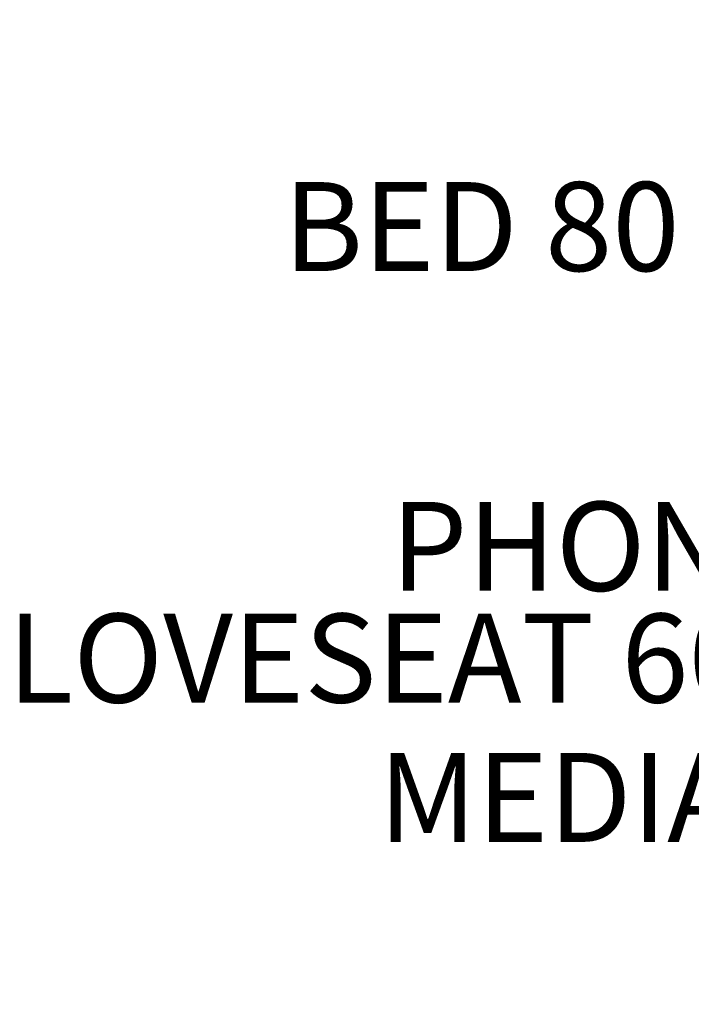
# Model space of a CAD drawing. Units: inches. Extents: x -307 to 2141, y -58 to 895.
# Tile 1 of 28: x -307 to 237, y -58 to 740. Entities that reach past the tile are written whole.
import ezdxf

# ---------------------------------------------------------------- set-up
doc = ezdxf.new("R2010")
doc.units = ezdxf.units.IN
doc.header["$MEASUREMENT"] = 0
doc.layers.add('A-ANNO-DIMS', color=2, linetype='Continuous', lineweight=18)
doc.styles.get("Standard").update_dxf_attribs({"font": 'arial.ttf'})
doc.dimstyles.get("Standard").update_dxf_attribs({"dimtxt": 72, "dimasz": 48, "dimexe": 0.18, "dimexo": 0.0625, "dimgap": 0.09, "dimtad": 0, "dimtih": 1, "dimtoh": 1, "dimdec": 0, "dimrnd": 48, "dimzin": 0, "dimdsep": 46, "dimlunit": 3, "dimtxsty": 'Standard', "dimcen": 0.09, "dimadec": 0, "dimazin": 0, "dimtfac": 1, "dimtdec": 0, "dimtofl": 0, "dimtmove": 0, "dimatfit": 3, "dimfxl": 1, "dimtolj": 1, "dimtzin": 0, "dimarcsym": 0})

# ---------------------------------------------------------------- blocks, each defined once
blk = doc.blocks.new('*D26')
at = {"layer": 'A-ANNO-DIMS', "color": 0, "lineweight": -2, "transparency": 16777216}
for p, q in [((565.34, 584.2), (565.34, 572.08)), ((645.34, 584.2), (645.34, 572.08)), ((517.34, 572.26), (469.34, 572.26)), ((693.34, 572.26), (741.34, 572.26))]:
    blk.add_line(p, q, dxfattribs=at)
at = {"layer": 'A-ANNO-DIMS', "color": 0, "transparency": 16777216}
for points in [[(517.34, 580.26), (517.34, 564.26), (565.34, 572.26)], [(693.34, 580.26), (693.34, 564.26), (645.34, 572.26)]]:
    blk.add_solid(points, dxfattribs=at)
at = {"layer": 'Defpoints', "color": 0, "transparency": 16777216}
for p in [(565.34, 584.26), (645.34, 584.26), (565.34, 572.26)]:
    blk.add_point(p, dxfattribs=at)
at = {"layer": 'A-ANNO-DIMS', "color": 0, "transparency": 16777216, "insert": (178.23, 572.26), "char_height": 72, "attachment_point": 5}
blk.add_mtext('\\A1;BED 80 TYP.', dxfattribs=at)
blk = doc.blocks.new('*D38')
at = {"layer": 'A-ANNO-DIMS', "color": 0, "lineweight": -2, "transparency": 16777216}
for p, q in [((598.5, 222.79), (550.5, 222.79)), ((646.5, 213.85), (646.5, 222.97)), ((706.5, 213.85), (706.5, 222.97)), ((754.5, 222.79), (802.5, 222.79))]:
    blk.add_line(p, q, dxfattribs=at)
at = {"layer": 'A-ANNO-DIMS', "color": 0, "transparency": 16777216}
for points in [[(598.5, 230.79), (598.5, 214.79), (646.5, 222.79)], [(754.5, 230.79), (754.5, 214.79), (706.5, 222.79)]]:
    blk.add_solid(points, dxfattribs=at)
at = {"layer": 'Defpoints', "color": 0, "transparency": 16777216}
for p in [(646.5, 222.79), (646.5, 213.79), (706.5, 213.79)]:
    blk.add_point(p, dxfattribs=at)
at = {"layer": 'A-ANNO-DIMS', "color": 0, "transparency": 16777216, "insert": (97.26, 222.79), "char_height": 72, "attachment_point": 5}
blk.add_mtext('\\A1;LOVESEAT 60 TYP.', dxfattribs=at)
blk = doc.blocks.new('*D48')
at = {"layer": 'A-ANNO-DIMS', "color": 0, "lineweight": -2, "transparency": 16777216}
for p, q in [((724, 313.98), (724, 361.98)), ((732.94, 265.98), (723.82, 265.98)), ((732.94, 205.98), (723.82, 205.98)), ((724, 157.98), (724, 109.98)), ((724, 109.98), (676, 109.98))]:
    blk.add_line(p, q, dxfattribs=at)
at = {"layer": 'A-ANNO-DIMS', "color": 0, "transparency": 16777216}
for points in [[(716, 313.98), (732, 313.98), (724, 265.98)], [(716, 157.98), (732, 157.98), (724, 205.98)]]:
    blk.add_solid(points, dxfattribs=at)
at = {"layer": 'Defpoints', "color": 0, "transparency": 16777216}
for p in [(733, 265.98), (724, 205.98), (733, 205.98)]:
    blk.add_point(p, dxfattribs=at)
at = {"layer": 'A-ANNO-DIMS', "color": 0, "transparency": 16777216, "insert": (321.56, 109.98), "char_height": 72, "attachment_point": 5}
blk.add_mtext('\\A1;MEDIA UNIT 60', dxfattribs=at)
blk = doc.blocks.new('*D50')
at = {"layer": 'A-ANNO-DIMS', "color": 0, "lineweight": -2, "transparency": 16777216}
for p, q in [((517.34, 313.33), (469.34, 313.33)), ((565.34, 315.8), (565.34, 313.15)), ((582.27, 315.8), (582.27, 313.15)), ((630.27, 313.33), (678.27, 313.33))]:
    blk.add_line(p, q, dxfattribs=at)
at = {"layer": 'A-ANNO-DIMS', "color": 0, "transparency": 16777216}
for points in [[(517.34, 321.33), (517.34, 305.33), (565.34, 313.33)], [(630.27, 321.33), (630.27, 305.33), (582.27, 313.33)]]:
    blk.add_solid(points, dxfattribs=at)
at = {"layer": 'Defpoints', "color": 0, "transparency": 16777216}
for p in [(565.34, 315.87), (565.34, 313.33), (582.27, 315.87)]:
    blk.add_point(p, dxfattribs=at)
at = {"layer": 'A-ANNO-DIMS', "color": 0, "transparency": 16777216, "insert": (226.65, 313.33), "char_height": 72, "attachment_point": 5}
blk.add_mtext('\\A1;PHONE 17', dxfattribs=at)

msp = doc.modelspace()

# ---------------------------------------------------------------- dimensions: what is measured, and where the dimension line sits
at = {"layer": 'A-ANNO-DIMS'}
for base, p1, p2, angle, text, picture, middle in [((565.3358, 572.2648), (645.3359, 584.2648), (565.3358, 584.2648), 180, 'BED <> TYP.', '*D26', (178.2254, 572.2648)), ((565.3358, 313.3263), (582.2714, 315.8666), (565.3358, 315.8666), 180, 'PHONE <>', '*D50', (226.651, 313.3263)), ((646.4965, 222.7908), (706.4965, 213.7908), (646.4965, 213.7908), 180, 'LOVESEAT <> TYP.', '*D38', (97.2632, 222.7908)), ((724.0025, 205.9815), (733.0025, 265.9815), (733.0025, 205.9815), 270, 'MEDIA UNIT <>', '*D48', (321.5605, 109.9815))]:
    dim = msp.add_linear_dim(base=base, p1=p1, p2=p2, angle=angle, text=text, dimstyle='Standard', override={"dimdec": 0, "dimlfac": 1, "dimrnd": 0, "dimzin": 0, "dimdsep": 46, "dimlunit": 2}, dxfattribs=at)
    dim.commit()
    dim.dimension.update_dxf_attribs({"geometry": picture, "text_midpoint": middle})

doc.saveas('drawing.dxf')
